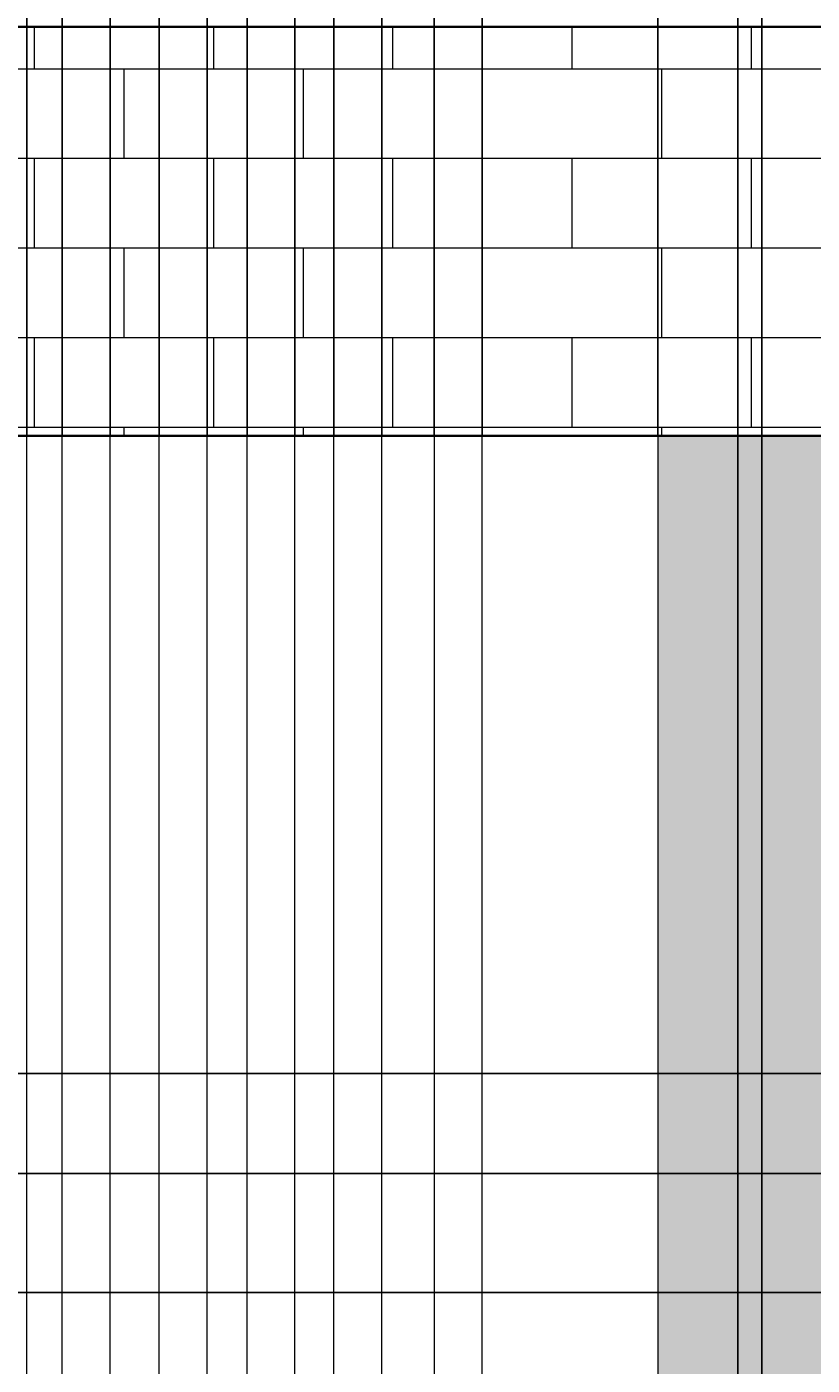
# Model space of a CAD drawing. Units: inches. Extents: x -13 to 809, y 112 to 656.
# Tile 37 of 55: x 389 to 455, y 446 to 559. Entities that reach past the tile are written whole.
import ezdxf

# ---------------------------------------------------------------- set-up
doc = ezdxf.new("R2010")
doc.units = ezdxf.units.IN
doc.header["$MEASUREMENT"] = 0
for name, color, linetype, lineweight in [('A-ANNO-DIMS', 2, 'Continuous', 18), ('A-ELEV', 7, 'Continuous', 35), ('A-ELEV-PATT', 8, 'Continuous', 13)]:
    doc.layers.add(name, color=color, linetype=linetype, lineweight=lineweight)
doc.styles.get("Standard").update_dxf_attribs({"font": 'arial.ttf'})
doc.dimstyles.get("Standard").update_dxf_attribs({"dimtxt": 0.625, "dimasz": 0.18, "dimexe": 0.18, "dimexo": 0.0625, "dimgap": 0.09, "dimtad": 0, "dimtih": 1, "dimtoh": 1, "dimdec": 4, "dimzin": 0, "dimdsep": 46, "dimlunit": 4, "dimtxsty": 'Standard', "dimcen": 0.09, "dimadec": 0, "dimazin": 0, "dimtfac": 1, "dimtdec": 4, "dimtofl": 0, "dimtmove": 0, "dimatfit": 3, "dimfxl": 1, "dimtolj": 1, "dimtzin": 0, "dimarcsym": 0})

# ---------------------------------------------------------------- blocks, each defined once
blk = doc.blocks.new('*D26')
at = {"layer": 'A-ANNO-DIMS', "color": 0, "lineweight": -2, "transparency": 16777216}
for p, q in [((341.41, 524.34), (341.41, 655.96)), ((341.59, 655.78), (405.14, 655.78)), ((470.92, 655.78), (407.37, 655.78)), ((471.1, 470.94), (471.1, 655.96))]:
    blk.add_line(p, q, dxfattribs=at)
at = {"layer": 'A-ANNO-DIMS', "color": 0, "transparency": 16777216}
for points in [[(341.59, 655.81), (341.59, 655.75), (341.41, 655.78)], [(470.92, 655.81), (470.92, 655.75), (471.1, 655.78)]]:
    blk.add_solid(points, dxfattribs=at)
at = {"layer": 'Defpoints', "color": 0, "transparency": 16777216}
for p in [(471.1, 655.78), (341.41, 524.28), (471.1, 470.88)]:
    blk.add_point(p, dxfattribs=at)
at = {"layer": 'A-ANNO-DIMS', "color": 0, "transparency": 16777216, "insert": (406.25, 655.78), "char_height": 0.625, "attachment_point": 5}
blk.add_mtext('\\A1;129.7', dxfattribs=at)
blk = doc.blocks.new('*D43')
at = {"layer": 'A-ANNO-DIMS', "color": 0, "lineweight": -2, "transparency": 16777216}
for p, q in [((471.04, 470.88), (-12.1, 470.88)), ((-11.92, 470.7), (-11.92, 443.28)), ((-11.92, 415.04), (-11.92, 442.46)), ((471.04, 414.86), (-12.1, 414.86))]:
    blk.add_line(p, q, dxfattribs=at)
at = {"layer": 'A-ANNO-DIMS', "color": 0, "transparency": 16777216}
for points in [[(-11.95, 470.7), (-11.89, 470.7), (-11.92, 470.88)], [(-11.95, 415.04), (-11.89, 415.04), (-11.92, 414.86)]]:
    blk.add_solid(points, dxfattribs=at)
at = {"layer": 'Defpoints', "color": 0, "transparency": 16777216}
for p in [(-11.92, 470.88), (471.1, 470.88), (471.1, 414.86)]:
    blk.add_point(p, dxfattribs=at)
at = {"layer": 'A-ANNO-DIMS', "color": 0, "transparency": 16777216, "insert": (-11.92, 442.87), "char_height": 0.625, "attachment_point": 5}
blk.add_mtext('\\A1;56.02', dxfattribs=at)
blk = doc.blocks.new('*D63')
at = {"layer": 'A-ANNO-DIMS', "color": 0, "lineweight": -2, "transparency": 16777216}
for p, q in [((389.35, 524.34), (389.35, 655.96)), ((389.53, 655.78), (389.69, 655.78)), ((392.15, 655.78), (391.99, 655.78)), ((392.33, 524.34), (392.33, 655.96))]:
    blk.add_line(p, q, dxfattribs=at)
at = {"layer": 'A-ANNO-DIMS', "color": 0, "transparency": 16777216}
for points in [[(389.53, 655.81), (389.53, 655.75), (389.35, 655.78)], [(392.15, 655.81), (392.15, 655.75), (392.33, 655.78)]]:
    blk.add_solid(points, dxfattribs=at)
at = {"layer": 'Defpoints', "color": 0, "transparency": 16777216}
for p in [(392.33, 655.78), (389.35, 524.28), (392.33, 524.28)]:
    blk.add_point(p, dxfattribs=at)
at = {"layer": 'A-ANNO-DIMS', "color": 0, "transparency": 16777216, "insert": (390.84, 655.78), "char_height": 0.625, "attachment_point": 5}
blk.add_mtext('\\A1;2.974', dxfattribs=at)
blk = doc.blocks.new('*D64')
at = {"layer": 'A-ANNO-DIMS', "color": 0, "lineweight": -2, "transparency": 16777216}
for p, q in [((392.33, 524.34), (392.33, 655.96)), ((392.51, 655.78), (394.02, 655.78)), ((396.15, 655.78), (394.63, 655.78)), ((396.33, 524.34), (396.33, 655.96))]:
    blk.add_line(p, q, dxfattribs=at)
at = {"layer": 'A-ANNO-DIMS', "color": 0, "transparency": 16777216}
for points in [[(392.51, 655.81), (392.51, 655.75), (392.33, 655.78)], [(396.15, 655.81), (396.15, 655.75), (396.33, 655.78)]]:
    blk.add_solid(points, dxfattribs=at)
at = {"layer": 'Defpoints', "color": 0, "transparency": 16777216}
for p in [(396.33, 655.78), (392.33, 524.28), (396.33, 524.28)]:
    blk.add_point(p, dxfattribs=at)
at = {"layer": 'A-ANNO-DIMS', "color": 0, "transparency": 16777216, "insert": (394.33, 655.78), "char_height": 0.625, "attachment_point": 5}
blk.add_mtext('\\A1;4', dxfattribs=at)
blk = doc.blocks.new('*D65')
at = {"layer": 'A-ANNO-DIMS', "color": 0, "lineweight": -2, "transparency": 16777216}
for p, q in [((396.33, 524.34), (396.33, 655.96)), ((396.51, 655.78), (397.48, 655.78)), ((400.27, 655.78), (399.3, 655.78)), ((400.45, 524.34), (400.45, 655.96))]:
    blk.add_line(p, q, dxfattribs=at)
at = {"layer": 'A-ANNO-DIMS', "color": 0, "transparency": 16777216}
for points in [[(396.51, 655.81), (396.51, 655.75), (396.33, 655.78)], [(400.27, 655.81), (400.27, 655.75), (400.45, 655.78)]]:
    blk.add_solid(points, dxfattribs=at)
at = {"layer": 'Defpoints', "color": 0, "transparency": 16777216}
for p in [(400.45, 655.78), (396.33, 524.28), (400.45, 524.28)]:
    blk.add_point(p, dxfattribs=at)
at = {"layer": 'A-ANNO-DIMS', "color": 0, "transparency": 16777216, "insert": (398.39, 655.78), "char_height": 0.625, "attachment_point": 5}
blk.add_mtext('\\A1;4.12', dxfattribs=at)
blk = doc.blocks.new('*D66')
at = {"layer": 'A-ANNO-DIMS', "color": 0, "lineweight": -2, "transparency": 16777216}
for p, q in [((400.45, 524.34), (400.45, 655.96)), ((400.63, 655.78), (402.14, 655.78)), ((404.27, 655.78), (402.75, 655.78)), ((404.45, 524.34), (404.45, 655.96))]:
    blk.add_line(p, q, dxfattribs=at)
at = {"layer": 'A-ANNO-DIMS', "color": 0, "transparency": 16777216}
for points in [[(400.63, 655.81), (400.63, 655.75), (400.45, 655.78)], [(404.27, 655.81), (404.27, 655.75), (404.45, 655.78)]]:
    blk.add_solid(points, dxfattribs=at)
at = {"layer": 'Defpoints', "color": 0, "transparency": 16777216}
for p in [(404.45, 655.78), (400.45, 524.28), (404.45, 524.28)]:
    blk.add_point(p, dxfattribs=at)
at = {"layer": 'A-ANNO-DIMS', "color": 0, "transparency": 16777216, "insert": (402.45, 655.78), "char_height": 0.625, "attachment_point": 5}
blk.add_mtext('\\A1;4', dxfattribs=at)
blk = doc.blocks.new('*D67')
at = {"layer": 'A-ANNO-DIMS', "color": 0, "lineweight": -2, "transparency": 16777216}
for p, q in [((404.45, 524.34), (404.45, 655.96)), ((404.63, 655.78), (404.98, 655.78)), ((407.62, 655.78), (407.27, 655.78)), ((407.8, 524.34), (407.8, 655.96))]:
    blk.add_line(p, q, dxfattribs=at)
at = {"layer": 'A-ANNO-DIMS', "color": 0, "transparency": 16777216}
for points in [[(404.63, 655.81), (404.63, 655.75), (404.45, 655.78)], [(407.62, 655.81), (407.62, 655.75), (407.8, 655.78)]]:
    blk.add_solid(points, dxfattribs=at)
at = {"layer": 'Defpoints', "color": 0, "transparency": 16777216}
for p in [(407.8, 655.78), (404.45, 524.28), (407.8, 524.28)]:
    blk.add_point(p, dxfattribs=at)
at = {"layer": 'A-ANNO-DIMS', "color": 0, "transparency": 16777216, "insert": (406.13, 655.78), "char_height": 0.625, "attachment_point": 5}
blk.add_mtext('\\A1;3.356', dxfattribs=at)
blk = doc.blocks.new('*D68')
at = {"layer": 'A-ANNO-DIMS', "color": 0, "lineweight": -2, "transparency": 16777216}
for p, q in [((407.8, 524.34), (407.8, 655.96)), ((407.98, 655.78), (409.5, 655.78)), ((411.62, 655.78), (410.11, 655.78)), ((411.8, 524.34), (411.8, 655.96))]:
    blk.add_line(p, q, dxfattribs=at)
at = {"layer": 'A-ANNO-DIMS', "color": 0, "transparency": 16777216}
for points in [[(407.98, 655.81), (407.98, 655.75), (407.8, 655.78)], [(411.62, 655.81), (411.62, 655.75), (411.8, 655.78)]]:
    blk.add_solid(points, dxfattribs=at)
at = {"layer": 'Defpoints', "color": 0, "transparency": 16777216}
for p in [(411.8, 655.78), (407.8, 524.28), (411.8, 524.28)]:
    blk.add_point(p, dxfattribs=at)
at = {"layer": 'A-ANNO-DIMS', "color": 0, "transparency": 16777216, "insert": (409.8, 655.78), "char_height": 0.625, "attachment_point": 5}
blk.add_mtext('\\A1;4', dxfattribs=at)
blk = doc.blocks.new('*D69')
at = {"layer": 'A-ANNO-DIMS', "color": 0, "lineweight": -2, "transparency": 16777216}
for p, q in [((411.8, 524.34), (411.8, 655.96)), ((411.98, 655.78), (412.35, 655.78)), ((414.89, 655.78), (414.52, 655.78)), ((415.07, 524.34), (415.07, 655.96))]:
    blk.add_line(p, q, dxfattribs=at)
at = {"layer": 'A-ANNO-DIMS', "color": 0, "transparency": 16777216}
for points in [[(411.98, 655.81), (411.98, 655.75), (411.8, 655.78)], [(414.89, 655.81), (414.89, 655.75), (415.07, 655.78)]]:
    blk.add_solid(points, dxfattribs=at)
at = {"layer": 'Defpoints', "color": 0, "transparency": 16777216}
for p in [(415.07, 655.78), (411.8, 524.28), (415.07, 524.28)]:
    blk.add_point(p, dxfattribs=at)
at = {"layer": 'A-ANNO-DIMS', "color": 0, "transparency": 16777216, "insert": (413.43, 655.78), "char_height": 0.625, "attachment_point": 5}
blk.add_mtext('\\A1;3.261', dxfattribs=at)
blk = doc.blocks.new('*D70')
at = {"layer": 'A-ANNO-DIMS', "color": 0, "lineweight": -2, "transparency": 16777216}
for p, q in [((415.07, 524.34), (415.07, 655.96)), ((415.25, 655.78), (416.76, 655.78)), ((418.89, 655.78), (417.37, 655.78)), ((419.07, 524.34), (419.07, 655.96))]:
    blk.add_line(p, q, dxfattribs=at)
at = {"layer": 'A-ANNO-DIMS', "color": 0, "transparency": 16777216}
for points in [[(415.25, 655.81), (415.25, 655.75), (415.07, 655.78)], [(418.89, 655.81), (418.89, 655.75), (419.07, 655.78)]]:
    blk.add_solid(points, dxfattribs=at)
at = {"layer": 'Defpoints', "color": 0, "transparency": 16777216}
for p in [(419.07, 655.78), (415.07, 524.28), (419.07, 524.28)]:
    blk.add_point(p, dxfattribs=at)
at = {"layer": 'A-ANNO-DIMS', "color": 0, "transparency": 16777216, "insert": (417.07, 655.78), "char_height": 0.625, "attachment_point": 5}
blk.add_mtext('\\A1;4', dxfattribs=at)
blk = doc.blocks.new('*D71')
at = {"layer": 'A-ANNO-DIMS', "color": 0, "lineweight": -2, "transparency": 16777216}
for p, q in [((419.07, 524.34), (419.07, 655.96)), ((419.25, 655.78), (420.11, 655.78)), ((423.29, 655.78), (422.43, 655.78)), ((423.47, 524.34), (423.47, 655.96))]:
    blk.add_line(p, q, dxfattribs=at)
at = {"layer": 'A-ANNO-DIMS', "color": 0, "transparency": 16777216}
for points in [[(419.25, 655.81), (419.25, 655.75), (419.07, 655.78)], [(423.29, 655.81), (423.29, 655.75), (423.47, 655.78)]]:
    blk.add_solid(points, dxfattribs=at)
at = {"layer": 'Defpoints', "color": 0, "transparency": 16777216}
for p in [(423.47, 655.78), (419.07, 524.28), (423.47, 524.28)]:
    blk.add_point(p, dxfattribs=at)
at = {"layer": 'A-ANNO-DIMS', "color": 0, "transparency": 16777216, "insert": (421.27, 655.78), "char_height": 0.625, "attachment_point": 5}
blk.add_mtext('\\A1;4.407', dxfattribs=at)
blk = doc.blocks.new('*D72')
at = {"layer": 'A-ANNO-DIMS', "color": 0, "lineweight": -2, "transparency": 16777216}
for p, q in [((423.47, 524.34), (423.47, 655.96)), ((423.65, 655.78), (425.17, 655.78)), ((427.29, 655.78), (425.78, 655.78)), ((427.47, 524.34), (427.47, 655.96))]:
    blk.add_line(p, q, dxfattribs=at)
at = {"layer": 'A-ANNO-DIMS', "color": 0, "transparency": 16777216}
for points in [[(423.65, 655.81), (423.65, 655.75), (423.47, 655.78)], [(427.29, 655.81), (427.29, 655.75), (427.47, 655.78)]]:
    blk.add_solid(points, dxfattribs=at)
at = {"layer": 'Defpoints', "color": 0, "transparency": 16777216}
for p in [(427.47, 655.78), (423.47, 524.28), (427.47, 524.28)]:
    blk.add_point(p, dxfattribs=at)
at = {"layer": 'A-ANNO-DIMS', "color": 0, "transparency": 16777216, "insert": (425.47, 655.78), "char_height": 0.625, "attachment_point": 5}
blk.add_mtext('\\A1;4', dxfattribs=at)
blk = doc.blocks.new('*D73')
at = {"layer": 'A-ANNO-DIMS', "color": 0, "lineweight": -2, "transparency": 16777216}
for p, q in [((427.47, 524.34), (427.47, 655.96)), ((427.65, 655.78), (433.47, 655.78)), ((442, 655.78), (436.18, 655.78)), ((442.18, 524.34), (442.18, 655.96))]:
    blk.add_line(p, q, dxfattribs=at)
at = {"layer": 'A-ANNO-DIMS', "color": 0, "transparency": 16777216}
for points in [[(427.65, 655.81), (427.65, 655.75), (427.47, 655.78)], [(442, 655.81), (442, 655.75), (442.18, 655.78)]]:
    blk.add_solid(points, dxfattribs=at)
at = {"layer": 'Defpoints', "color": 0, "transparency": 16777216}
for p in [(442.18, 655.78), (427.47, 524.28), (442.18, 524.28)]:
    blk.add_point(p, dxfattribs=at)
at = {"layer": 'A-ANNO-DIMS', "color": 0, "transparency": 16777216, "insert": (434.83, 655.78), "char_height": 0.625, "attachment_point": 5}
blk.add_mtext('\\A1;14.712', dxfattribs=at)
blk = doc.blocks.new('*D104')
at = {"layer": 'A-ANNO-DIMS', "color": 0, "lineweight": -2, "transparency": 16777216}
for p, q in [((337.57, 462.52), (807.77, 462.52)), ((807.59, 462.34), (807.59, 457.95)), ((807.59, 452.74), (807.59, 457.13)), ((319.76, 452.56), (807.77, 452.56))]:
    blk.add_line(p, q, dxfattribs=at)
at = {"layer": 'A-ANNO-DIMS', "color": 0, "transparency": 16777216}
for points in [[(807.56, 462.34), (807.62, 462.34), (807.59, 462.52)], [(807.56, 452.74), (807.62, 452.74), (807.59, 452.56)]]:
    blk.add_solid(points, dxfattribs=at)
at = {"layer": 'Defpoints', "color": 0, "transparency": 16777216}
for p in [(337.51, 462.52), (319.7, 452.56), (807.59, 452.56)]:
    blk.add_point(p, dxfattribs=at)
at = {"layer": 'A-ANNO-DIMS', "color": 0, "transparency": 16777216, "insert": (807.59, 457.54), "char_height": 0.625, "attachment_point": 5}
blk.add_mtext('\\A1;9.957', dxfattribs=at)
blk = doc.blocks.new('*D105')
at = {"layer": 'A-ANNO-DIMS', "color": 0, "lineweight": -2, "transparency": 16777216}
for p, q in [((319.76, 452.56), (807.77, 452.56)), ((807.59, 452.38), (807.59, 448.95)), ((807.59, 444.7), (807.59, 448.13)), ((319.57, 444.52), (807.77, 444.52))]:
    blk.add_line(p, q, dxfattribs=at)
at = {"layer": 'A-ANNO-DIMS', "color": 0, "transparency": 16777216}
for points in [[(807.56, 452.38), (807.62, 452.38), (807.59, 452.56)], [(807.56, 444.7), (807.62, 444.7), (807.59, 444.52)]]:
    blk.add_solid(points, dxfattribs=at)
at = {"layer": 'Defpoints', "color": 0, "transparency": 16777216}
for p in [(319.7, 452.56), (319.51, 444.52), (807.59, 444.52)]:
    blk.add_point(p, dxfattribs=at)
at = {"layer": 'A-ANNO-DIMS', "color": 0, "transparency": 16777216, "insert": (807.59, 448.54), "char_height": 0.625, "attachment_point": 5}
blk.add_mtext('\\A1;8.043', dxfattribs=at)
blk = doc.blocks.new('*D133')
at = {"layer": 'A-ANNO-DIMS', "color": 0, "lineweight": -2, "transparency": 16777216}
for p, q in [((448.701738, 655.782835), (448.521738, 655.782835)), ((448.881738, 207.535185), (448.881738, 655.962835)), ((450.881738, 207.527657), (450.881738, 655.962835)), ((451.061738, 655.782835), (451.241738, 655.782835))]:
    blk.add_line(p, q, dxfattribs=at)
at = {"layer": 'A-ANNO-DIMS', "color": 0, "transparency": 16777216}
for points in [[(448.701738, 655.812835), (448.701738, 655.752835), (448.881738, 655.782835)], [(451.061738, 655.812835), (451.061738, 655.752835), (450.881738, 655.782835)]]:
    blk.add_solid(points, dxfattribs=at)
at = {"layer": 'Defpoints', "color": 0, "transparency": 16777216}
for p in [(450.881738, 655.782835), (448.881738, 207.472685), (450.881738, 207.465157)]:
    blk.add_point(p, dxfattribs=at)
at = {"layer": 'A-ANNO-DIMS', "color": 0, "transparency": 16777216, "insert": (449.881738, 655.782835), "char_height": 0.625, "attachment_point": 5}
blk.add_mtext('\\A1;2.00', dxfattribs=at)

msp = doc.modelspace()

# ---------------------------------------------------------------- hatches: boundary and pattern name
at = {"layer": 'A-ELEV-PATT'}
h = msp.add_hatch(dxfattribs=at)
h.set_pattern_fill('BRICK', color=256, scale=30)
h.paths.add_polyline_path([(591.008, 558.5199), (341.4072, 558.5199), (341.4072, 524.281), (542.9617, 524.281), (542.9617, 288.4508), (341.4072, 288.4508), (341.4072, 250.8429), (591.008, 250.8429)])
h = msp.add_hatch(dxfattribs=at)
h.set_pattern_fill('CROSS', color=256, scale=9.7)
h.paths.add_polyline_path([(542.9617, 524.281), (442.1845, 524.281), (442.1845, 288.4508), (542.9617, 288.4508)])
h.paths.add_polyline_path([(471.0998, 470.8765), (471.0998, 498.1452), (510.462, 498.1452), (510.462, 470.8765)], flags=16)
h.paths.add_polyline_path([(473.0998, 472.8765), (473.0998, 496.1452), (508.462, 496.1452), (508.462, 472.8765)], flags=0)
h.paths.add_polyline_path([(471.0998, 442.128), (510.462, 442.128), (510.462, 414.8594), (471.0998, 414.8594)], flags=16)
h.paths.add_polyline_path([(473.0998, 440.128), (508.462, 440.128), (508.462, 416.8594), (473.0998, 416.8594)], flags=0)
h.paths.add_polyline_path([(471.0998, 385.2491), (510.462, 385.2491), (510.462, 357.9804), (471.0998, 357.9804)], flags=16)
h.paths.add_polyline_path([(473.0998, 383.2491), (508.462, 383.2491), (508.462, 359.9804), (473.0998, 359.9804)], flags=0)
h.paths.add_polyline_path([(471.0998, 340.4353), (510.462, 340.4353), (510.462, 313.1667), (471.0998, 313.1667)], flags=16)
h.paths.add_polyline_path([(473.0998, 338.4353), (508.462, 338.4353), (508.462, 315.1667), (473.0998, 315.1667)], flags=0)

# ---------------------------------------------------------------- linework, layer by layer
at = {"layer": 'A-ELEV'}
msp.add_line((341.4072, 558.5199), (591.008, 558.5199), dxfattribs=at)
for points in [[(341.4072, 558.5199), (591.008, 558.5199), (591.008, 250.8429), (341.4072, 250.8429)], [(341.4072, 524.281), (542.9617, 524.281), (542.9617, 288.4508), (341.4072, 288.4508)]]:
    msp.add_lwpolyline(points, close=True, dxfattribs=at)
at = {"layer": 'A-ELEV-PATT'}
msp.add_line((442.1845, 524.281), (442.1845, 288.4508), dxfattribs=at)
for points in [[(389.3536, 288.4508), (389.3536, 523.3908), (389.3536, 524.281)], [(392.3277, 288.4508), (392.3277, 523.3908), (392.3277, 524.281)], [(396.3277, 288.4508), (396.3277, 523.3908), (396.3277, 524.281)], [(400.4483, 288.4508), (400.4483, 523.3908), (400.4483, 524.281)], [(404.4483, 288.4508), (404.4483, 523.3908), (404.4483, 524.281)], [(407.8046, 288.4508), (407.8046, 523.3908), (407.8046, 524.281)], [(411.8046, 288.4508), (411.8046, 523.3908), (411.8046, 524.281)], [(415.0653, 288.4508), (415.0653, 523.3908), (415.0653, 524.281)], [(419.0653, 288.4508), (419.0653, 523.3908), (419.0653, 524.281)], [(423.4725, 288.4508), (423.4725, 523.3908), (423.4725, 524.281)], [(427.4725, 288.4508), (427.4725, 523.3908), (427.4725, 524.281)]]:
    msp.add_lwpolyline(points, dxfattribs=at)

# ---------------------------------------------------------------- dimensions: what is measured, and where the dimension line sits
at = {"layer": 'A-ANNO-DIMS'}
for base, p1, p2, override, picture, middle in [((471.0998, 655.7828), (341.4072, 524.281), (471.0998, 470.8765), {"dimdec": 1, "dimlfac": 1, "dimrnd": 0, "dimzin": 0, "dimdsep": 46, "dimlunit": 2}, '*D26', (406.2535, 655.7828)), ((392.3277, 655.7828), (389.3536, 524.281), (392.3277, 524.281), {"dimdec": 3, "dimlfac": 1, "dimrnd": 0, "dimzin": 0, "dimdsep": 46, "dimlunit": 2}, '*D63', (390.8407, 655.7828)), ((396.3277, 655.7828), (392.3277, 524.281), (396.3277, 524.281), {"dimdec": 0, "dimlfac": 1, "dimrnd": 0, "dimzin": 0, "dimdsep": 46, "dimlunit": 2}, '*D64', (394.3277, 655.7828)), ((400.4483, 655.7828), (396.3277, 524.281), (400.4483, 524.281), {"dimdec": 2, "dimlfac": 1, "dimrnd": 0, "dimzin": 0, "dimdsep": 46, "dimlunit": 2}, '*D65', (398.388, 655.7828)), ((404.4483, 655.7828), (400.4483, 524.281), (404.4483, 524.281), {"dimdec": 0, "dimlfac": 1, "dimrnd": 0, "dimzin": 0, "dimdsep": 46, "dimlunit": 2}, '*D66', (402.4483, 655.7828)), ((407.8046, 655.7828), (404.4483, 524.281), (407.8046, 524.281), {"dimdec": 3, "dimlfac": 1, "dimrnd": 0, "dimzin": 0, "dimdsep": 46, "dimlunit": 2}, '*D67', (406.1264, 655.7828)), ((411.8046, 655.7828), (407.8046, 524.281), (411.8046, 524.281), {"dimdec": 0, "dimlfac": 1, "dimrnd": 0, "dimzin": 0, "dimdsep": 46, "dimlunit": 2}, '*D68', (409.8046, 655.7828)), ((415.0653, 655.7828), (411.8046, 524.281), (415.0653, 524.281), {"dimdec": 3, "dimlfac": 1, "dimrnd": 0, "dimzin": 0, "dimdsep": 46, "dimlunit": 2}, '*D69', (413.4349, 655.7828)), ((419.0653, 655.7828), (415.0653, 524.281), (419.0653, 524.281), {"dimdec": 0, "dimlfac": 1, "dimrnd": 0, "dimzin": 0, "dimdsep": 46, "dimlunit": 2}, '*D70', (417.0653, 655.7828)), ((423.4725, 655.7828), (419.0653, 524.281), (423.4725, 524.281), {"dimdec": 3, "dimlfac": 1, "dimrnd": 0, "dimzin": 0, "dimdsep": 46, "dimlunit": 2}, '*D71', (421.2689, 655.7828)), ((427.4725, 655.7828), (423.4725, 524.281), (427.4725, 524.281), {"dimdec": 0, "dimlfac": 1, "dimrnd": 0, "dimzin": 0, "dimdsep": 46, "dimlunit": 2}, '*D72', (425.4725, 655.7828)), ((442.1845, 655.7828), (427.4725, 524.281), (442.1845, 524.281), {"dimdec": 3, "dimlfac": 1, "dimrnd": 0, "dimzin": 0, "dimdsep": 46, "dimlunit": 2}, '*D73', (434.8285, 655.7828)), ((450.8817, 655.7828), (448.8817, 207.4727), (450.8817, 207.4652), {"dimdec": 2, "dimlfac": 1, "dimrnd": 0, "dimzin": 0, "dimdsep": 46, "dimlunit": 2}, '*D133', (449.8817, 655.7828))]:
    dim = msp.add_linear_dim(base=base, p1=p1, p2=p2, dimstyle='Standard', override=override, dxfattribs=at)
    dim.commit()
    dim.dimension.update_dxf_attribs({"geometry": picture, "text_midpoint": middle})
for base, p1, p2, override, picture, middle in [((-11.9191, 470.8765), (471.0998, 414.8594), (471.0998, 470.8765), {"dimdec": 2, "dimlfac": 1, "dimrnd": 0, "dimzin": 0, "dimdsep": 46, "dimlunit": 2}, '*D43', (-11.9191, 442.8679)), ((807.5888, 452.5629), (337.5074, 462.5199), (319.7004, 452.5629), {"dimdec": 3, "dimlfac": 1, "dimrnd": 0, "dimzin": 0, "dimdsep": 46, "dimlunit": 2}, '*D104', (807.5888, 457.5414)), ((807.5888, 444.5199), (319.7004, 452.5629), (319.5074, 444.5199), {"dimdec": 3, "dimlfac": 1, "dimrnd": 0, "dimzin": 0, "dimdsep": 46, "dimlunit": 2}, '*D105', (807.5888, 448.5414))]:
    dim = msp.add_linear_dim(base=base, p1=p1, p2=p2, angle=90, dimstyle='Standard', override=override, dxfattribs=at)
    dim.commit()
    dim.dimension.update_dxf_attribs({"geometry": picture, "text_midpoint": middle})

doc.saveas('drawing.dxf')
